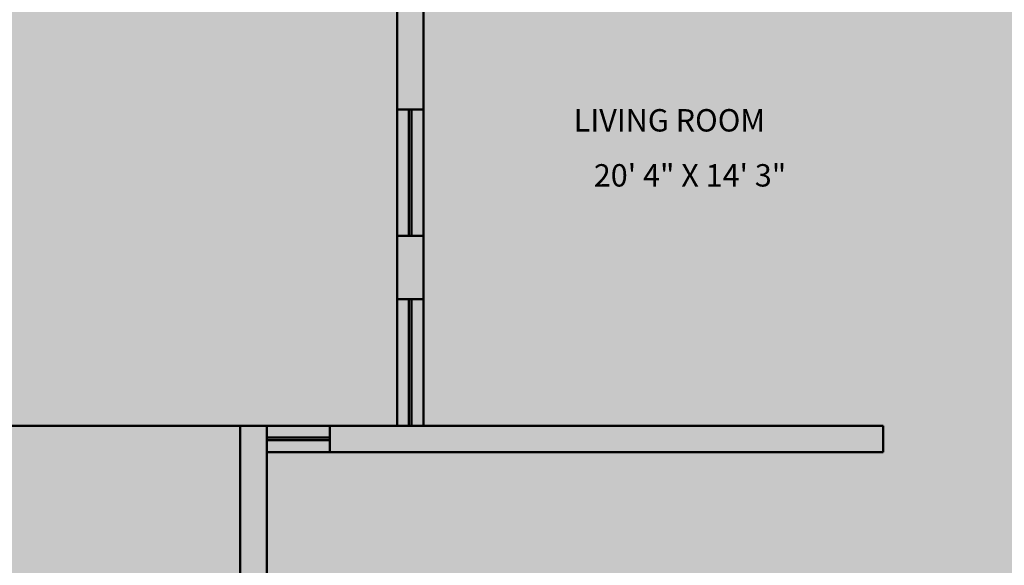
# Model space of a CAD drawing. Units: inches. Extents: x 925 to 2834, y 111 to 1355.
# Tile 4 of 25: x 1116 to 1490, y 675 to 882. Entities that reach past the tile are written whole.
import ezdxf

# ---------------------------------------------------------------- set-up
doc = ezdxf.new("R2010")
doc.units = ezdxf.units.IN
doc.header["$MEASUREMENT"] = 0
for name, color, linetype, lineweight in [('A-ANNO-DIMS', 2, 'Continuous', 18), ('A-AREA-IDEN', 7, 'Continuous', 18), ('A-FLOR-PATT', 252, 'Continuous', 13), ('A-WALL', 7, 'Continuous', 50), ('A-WALL-PATT', 8, 'Continuous', 13)]:
    doc.layers.add(name, color=color, linetype=linetype, lineweight=lineweight)
doc.styles.get("Standard").update_dxf_attribs({"font": 'arial.ttf'})
doc.dimstyles.get("Standard").update_dxf_attribs({"dimtxt": 6, "dimasz": 3, "dimexe": 0.18, "dimexo": 0.0625, "dimgap": 0.09, "dimtad": 0, "dimtih": 1, "dimtoh": 1, "dimdec": 1, "dimzin": 0, "dimdsep": 46, "dimlunit": 3, "dimtxsty": 'Standard', "dimblk": 'ARCHTICK', "dimcen": 0.09, "dimadec": 0, "dimazin": 0, "dimtfac": 1, "dimtdec": 1, "dimtofl": 0, "dimtmove": 0, "dimatfit": 3, "dimfxl": 1, "dimtolj": 1, "dimtzin": 0, "dimarcsym": 0})

# ---------------------------------------------------------------- blocks, each defined once
blk = doc.blocks.new('_ArchTick')
at = {"color": 0, "linetype": 'ByBlock', "const_width": 0.15}
blk.add_lwpolyline([(-0.5, -0.5), (0.5, 0.5)], dxfattribs=at)
blk = doc.blocks.new('*D25')
at = {"layer": 'A-ANNO-DIMS', "color": 0, "lineweight": -2, "transparency": 16777216}
for p, q in [((1200.21, 727.53), (1200.21, 115.18)), ((1084.71, 265.03), (1084.71, 115.18)), ((1084.71, 115.36), (1132.51, 115.36)), ((1200.21, 115.36), (1152.42, 115.36))]:
    blk.add_line(p, q, dxfattribs=at)
at = {"layer": 'Defpoints', "color": 0, "transparency": 16777216}
for p in [(1200.21, 727.59), (1084.71, 265.09), (1200.21, 115.36)]:
    blk.add_point(p, dxfattribs=at)
at = {"layer": 'A-ANNO-DIMS', "color": 0, "lineweight": -2, "transparency": 16777216, "xscale": 3, "yscale": 3, "zscale": 3, "rotation": 180}
blk.add_blockref('_ArchTick', (1084.71, 115.36), dxfattribs=at)
at = {"layer": 'A-ANNO-DIMS', "color": 0, "lineweight": -2, "transparency": 16777216, "xscale": 3, "yscale": 3, "zscale": 3}
blk.add_blockref('_ArchTick', (1200.21, 115.36), dxfattribs=at)
at = {"layer": 'A-ANNO-DIMS', "color": 0, "transparency": 16777216, "insert": (1142.46, 115.36), "char_height": 6, "attachment_point": 5}
blk.add_mtext('\\A1;115.5', dxfattribs=at)
blk = doc.blocks.new('*D26')
at = {"layer": 'A-ANNO-DIMS', "color": 0, "lineweight": -2, "transparency": 16777216}
for p, q in [((1200.21, 727.53), (1200.21, 115.18)), ((1434.21, 385.03), (1434.21, 115.18)), ((1200.21, 115.36), (1310.46, 115.36)), ((1434.21, 115.36), (1323.97, 115.36))]:
    blk.add_line(p, q, dxfattribs=at)
at = {"layer": 'Defpoints', "color": 0, "transparency": 16777216}
for p in [(1200.21, 727.59), (1434.21, 385.09), (1434.21, 115.36)]:
    blk.add_point(p, dxfattribs=at)
at = {"layer": 'A-ANNO-DIMS', "color": 0, "lineweight": -2, "transparency": 16777216, "xscale": 3, "yscale": 3, "zscale": 3, "rotation": 180}
blk.add_blockref('_ArchTick', (1200.21, 115.36), dxfattribs=at)
at = {"layer": 'A-ANNO-DIMS', "color": 0, "lineweight": -2, "transparency": 16777216, "xscale": 3, "yscale": 3, "zscale": 3}
blk.add_blockref('_ArchTick', (1434.21, 115.36), dxfattribs=at)
at = {"layer": 'A-ANNO-DIMS', "color": 0, "transparency": 16777216, "insert": (1317.21, 115.36), "char_height": 6, "attachment_point": 5}
blk.add_mtext('\\A1;234', dxfattribs=at)

msp = doc.modelspace()

# ---------------------------------------------------------------- hatches: boundary and pattern name
at = {"layer": 'A-FLOR-PATT', "transparency": 33554605}
h = msp.add_hatch(color=256, dxfattribs=at)
h.dxf.hatch_style = 1
h.paths.add_polyline_path([(1931.688, 1294.5638), (991.7375, 1294.5638), (991.7375, 172.1134), (1931.688, 172.1134)])
h.paths.add_polyline_path([(1910.7128, 1273.5886), (1910.7128, 193.0886), (1012.7128, 193.0886), (1012.7128, 1273.5886)], flags=16)
h.paths.add_polyline_path([(1850.7128, 1213.5886), (1850.7128, 253.0886), (1072.7128, 253.0886), (1072.7128, 1213.5886)], flags=0)
h.paths.add_polyline_path([(1838.7128, 1201.5886), (1838.7128, 265.0886), (1084.7128, 265.0886), (1084.7128, 530.5886), (1084.7128, 1201.5886)], flags=0)
h.paths.add_polyline_path([(1547.6758, 1155.7396), (1547.6758, 1119.115), (1513.0687, 1119.115), (1513.0687, 1155.7396)], flags=0)
h.paths.add_polyline_path([(1600.1067, 1154.9439), (1634.7139, 1154.9439), (1634.7139, 1119.115), (1600.1067, 1119.115)], flags=0)
h.paths.add_polyline_path([(1505.2502, 1144.5358), (1505.2502, 1119.115), (1470.643, 1119.115), (1470.643, 1144.5358)], flags=0)
h.paths.add_polyline_path([(1559.1357, 1141.0962), (1593.7428, 1141.0962), (1593.7428, 1119.115), (1559.1357, 1119.115)], flags=0)
h.paths.add_polyline_path([(1462.8966, 1154.9439), (1462.8966, 1119.115), (1428.2895, 1119.115), (1428.2895, 1154.9439)], flags=0)
h.paths.add_polyline_path([(1642.4603, 1144.5358), (1677.0675, 1144.5358), (1677.0675, 1119.115), (1642.4603, 1119.115)], flags=0)
h.paths.add_polyline_path([(1422.3508, 1141.0962), (1422.3508, 1119.115), (1387.7436, 1119.115), (1387.7436, 1141.0962)], flags=0)
h.paths.add_polyline_path([(1684.8859, 1155.7396), (1719.4931, 1155.7396), (1719.4931, 1119.115), (1684.8859, 1119.115)], flags=0)
h.paths.add_polyline_path([(1718.7128, 1081.5886), (1718.7128, 1050.1249), (1715.7128, 1050.1249), (1715.7128, 1026.1249), (1715.7128, 1002.1249), (1718.7128, 1002.1249), (1730.7128, 1002.1249), (1730.7128, 998.1249), (1730.7128, 990.1249), (1730.7128, 986.1249), (1718.7128, 986.1249), (1718.7128, 893.5886), (1715.3735, 893.5886), (1715.3735, 891.5886), (1713.3735, 891.5886, 0.41421356), (1677.3735, 855.5886), (1713.3735, 855.5886), (1713.3735, 853.5886), (1715.3735, 853.5886), (1715.3735, 851.5886), (1718.7128, 851.5886), (1718.7128, 821.5865), (1734.4655, 821.5865), (1734.3735, 819.5886, -0.41421356), (1712.4415, 793.5886), (1712.4415, 791.5886), (1718.7128, 791.5886), (1718.7128, 717.5886), (1718.7128, 669.5886), (1732.7128, 669.5886), (1732.7128, 665.5886), (1732.7128, 641.5886), (1732.7128, 634.5886), (1732.7128, 610.5886), (1732.7128, 603.5886), (1718.7128, 603.5886), (1718.7128, 385.0886), (1434.2128, 385.0886), (1434.2128, 530.5886), (1410.2128, 530.5886), (1408.2128, 530.5886), (1408.2128, 532.5886, 0.41421356), (1372.2128, 568.5886), (1372.2128, 532.5886), (1370.2128, 532.5886), (1370.2128, 530.5886), (1368.2128, 530.5886), (1282.2128, 530.5886), (1210.2128, 530.5886), (1200.2128, 530.5886), (1200.2128, 542.1915), (1183.2307, 542.1915), (1183.2307, 546.1915), (1200.2128, 546.1915), (1200.2128, 572.1915), (1183.2307, 572.1915), (1183.2307, 576.1915), (1200.2128, 576.1915), (1200.2128, 727.5886), (1210.2128, 727.5886), (1234.2128, 727.5886), (1259.7128, 727.5886), (1259.7128, 775.5886), (1259.7128, 799.5886), (1259.7128, 847.5886), (1259.7128, 993.5872), (1259.7128, 1065.5872), (1259.7128, 1071.5886), (1219.6318, 1071.5886), (1219.6318, 1081.5886), (1084.7128, 1081.5886), (1084.7128, 1119.115), (1256.8974, 1119.115), (1256.8974, 1154.9439), (1291.5046, 1154.9439), (1291.5046, 1119.115), (1256.8974, 1119.115), (1256.6723, 1081.5886), (1293.7128, 1081.5886), (1341.7128, 1081.5886), (1341.7128, 1093.5886), (1347.7128, 1093.5886), (1371.7128, 1093.5886), (1377.7128, 1093.5886), (1377.7128, 1081.5886), (1668.7128, 1081.5886), (1668.7128, 1117.5886), (1675.7128, 1117.5886), (1711.7128, 1117.5886), (1718.7128, 1117.5886)], flags=0)
h.paths.add_polyline_path([(1376.2838, 1155.7396), (1376.2838, 1119.115), (1341.6766, 1119.115), (1341.6766, 1155.7396)], flags=0)
h.paths.add_polyline_path([(1341.7128, 1076.0886), (1293.7128, 1076.0886), (1293.7128, 1071.5886), (1269.7128, 1071.5886), (1269.7128, 1065.5872), (1266.7128, 1065.5872), (1266.7128, 1029.5872), (1265.7128, 1029.5872), (1265.7128, 993.5872), (1269.7128, 993.5872), (1269.7128, 903.5886), (1269.7128, 893.5886), (1269.7128, 847.5886), (1265.2128, 847.5886), (1265.2128, 799.5886), (1269.7128, 799.5886), (1269.7128, 775.5886), (1265.2128, 775.5886), (1265.2128, 727.5886), (1269.7128, 727.5886), (1444.2128, 727.5886), (1444.2128, 717.5886), (1234.2128, 717.5886), (1234.2128, 722.0886), (1210.2128, 722.0886), (1210.2128, 717.5886), (1210.2128, 540.5886), (1210.2128, 536.0886), (1282.2128, 536.0886), (1282.2128, 535.0886), (1210.2128, 535.0886), (1210.2128, 540.5886), (1210.2128, 717.5886), (1210.2128, 723.0886), (1234.2128, 723.0886), (1234.2128, 717.5886), (1444.2128, 717.5886), (1444.2128, 727.5886), (1269.7128, 727.5886), (1264.2128, 727.5886), (1264.2128, 775.5886), (1269.7128, 775.5886), (1269.7128, 799.5886), (1264.2128, 799.5886), (1264.2128, 847.5886), (1269.7128, 847.5886), (1269.7128, 893.5886), (1269.7128, 903.5886), (1269.7128, 993.5872), (1264.7128, 993.5872), (1264.7128, 1029.5872), (1265.7128, 1029.5872), (1265.7128, 1065.5872), (1269.7128, 1065.5872), (1269.7128, 1071.5886), (1293.7128, 1071.5886), (1293.7128, 1077.0886), (1341.7128, 1077.0886)], flags=0)
h.paths.add_polyline_path([(1730.9529, 1141.0962), (1765.5601, 1141.0962), (1765.5601, 1119.115), (1730.9529, 1119.115)], flags=0)
h.paths.add_polyline_path([(1333.8582, 1144.5358), (1333.8582, 1119.115), (1299.251, 1119.115), (1299.251, 1144.5358)], flags=0)
h.paths.add_polyline_path([(1592.7128, 968.5886), (1596.0342, 968.5886), (1602.7128, 968.5886), (1708.7128, 968.5886), (1708.7128, 903.5886), (1602.7128, 903.5886), (1602.7128, 938.5886), (1592.7128, 938.5886), (1592.7128, 903.5886), (1451.7128, 903.5886), (1451.7128, 893.5886), (1511.7128, 893.5886), (1511.7128, 881.5886), (1515.2128, 881.5886), (1518.7128, 881.5886), (1518.7128, 893.5886), (1592.7128, 893.5886), (1592.7128, 799.5886), (1518.7128, 799.5886), (1518.7128, 857.5886), (1511.7128, 857.5886), (1511.7128, 799.5886), (1511.7128, 772.0886), (1521.7128, 772.0886), (1521.7128, 792.5886), (1592.7128, 792.5886), (1592.7128, 727.5886), (1521.7128, 727.5886), (1521.7128, 748.0886), (1511.7128, 748.0886), (1511.7128, 717.5886), (1708.7128, 717.5886), (1714.2128, 717.5886), (1714.2128, 669.5886), (1708.7128, 669.5886), (1708.7128, 641.5886), (1492.2128, 641.5886), (1492.2128, 631.5886), (1621.2128, 631.5886), (1621.2128, 443.0886), (1625.7128, 443.0886), (1625.7128, 503.0886), (1625.7128, 507.5886), (1625.7128, 631.5886), (1708.7128, 631.5886), (1708.7128, 507.5886), (1655.7128, 507.5886), (1655.7128, 503.0886), (1708.7128, 503.0886), (1708.7128, 395.0886), (1625.7128, 395.0886), (1625.7128, 419.0886), (1621.2128, 419.0886), (1621.2128, 395.0886), (1482.2128, 395.0886), (1482.2128, 385.0886), (1434.2128, 385.0886), (1434.2128, 433.0886), (1444.2128, 433.0886), (1444.2128, 631.5886), (1450.2128, 631.5886), (1450.2128, 634.91), (1452.2128, 634.91), (1452.2128, 669.5886), (1454.2128, 669.5886, -0.40021217), (1490.1712, 635.3173), (1492.2128, 635.3173), (1492.2128, 641.5886), (1564.7128, 641.5886), (1564.7128, 677.5886), (1672.7128, 677.5886), (1672.7128, 681.5886), (1564.7128, 681.5886), (1564.7128, 717.5886), (1511.7128, 717.5886), (1511.7128, 748.0886), (1511.7128, 772.0886), (1511.7128, 799.5886), (1511.7128, 857.5886), (1511.8913, 857.5886), (1511.8913, 859.5886), (1515.6201, 859.5886, 0.41421356), (1537.552, 879.5886), (1513.552, 879.5886), (1511.8913, 879.5886), (1511.8913, 881.5886), (1511.7128, 881.5886), (1511.7128, 893.5886), (1451.7128, 893.5886), (1451.7128, 903.5886), (1592.7128, 903.5886), (1592.7128, 938.5886), (1592.7128, 940.5886), (1596.4415, 940.5886, 0.41421356), (1618.3735, 966.5886), (1594.3735, 966.5886), (1592.7128, 966.5886)], flags=0)
h.paths.add_polyline_path([(1377.7128, 903.5886), (1377.7128, 893.5886), (1305.7128, 893.5886), (1305.7128, 903.5886)], flags=0)
h.paths.add_polyline_path([(1708.7128, 821.5886), (1712.0342, 821.5886), (1712.0342, 819.5886), (1710.3735, 819.5886), (1708.7128, 819.5886)], flags=0)
h.paths.add_polyline_path([(1576.7128, 695.1992), (1575.5896, 693.6649), (1575.9687, 694.6994), (1575.4438, 695.1992), (1575.9687, 695.699), (1575.5896, 696.7335)], flags=0)
h.paths.add_polyline_path([(1565.9817, 662.3134), (1565.4568, 661.8136), (1565.8359, 660.7791), (1564.7128, 662.3134), (1565.8359, 663.8477), (1565.4568, 662.8132)], flags=0)
h.paths.add_polyline_path([(1444.2128, 433.0886), (1444.2128, 395.0886), (1482.2128, 395.0886), (1482.2128, 389.0886), (1438.2128, 389.0886), (1438.2128, 391.8608), (1438.2128, 433.0886)], flags=0)
h.paths.add_polyline_path([(1410.2128, 506.5886), (1410.2128, 289.0886), (1108.7128, 289.0886), (1108.7128, 506.5886)], flags=0)
h.paths.add_polyline_path([(1612.3153, 838.3016), (1680.4151, 838.3016), (1680.4151, 851.3131), (1612.3153, 851.3131)], flags=8)
h.paths.add_polyline_path([(1208.3174, 395.0436), (1282.1017, 395.0436), (1282.1017, 408.0552), (1208.3174, 408.0552)], flags=8)
h.paths.add_polyline_path([(1291.8049, 598.7427), (1369.8017, 598.7427), (1369.8017, 611.7542), (1291.8049, 611.7542)], flags=8)
h.paths.add_polyline_path([(1119.679, 917.3022), (1191.0817, 917.3022), (1191.0817, 930.3137), (1119.679, 930.3137)], flags=8)
h.paths.add_polyline_path([(1332.2261, 815.9808), (1410.2258, 815.9808), (1410.2258, 829.001), (1332.2261, 829.001)], flags=8)
h.paths.add_polyline_path([(1390.9013, 955.8158), (1475.4981, 955.8158), (1475.4981, 968.8273), (1390.9013, 968.8273)], flags=8)
h.paths.add_polyline_path([(1620.3436, 998.9325), (1688.4434, 998.9325), (1688.4434, 1011.944), (1620.3436, 1011.944)], flags=8)
h.paths.add_polyline_path([(1620.3436, 914.1039), (1691.7405, 914.1039), (1691.7405, 927.1155), (1620.3436, 927.1155)], flags=8)
h.paths.add_polyline_path([(1521.4542, 816.005), (1589.5569, 816.005), (1589.5569, 829.0253), (1521.4542, 829.0253)], flags=8)
h.paths.add_polyline_path([(1528.524, 740.3497), (1602.3082, 740.3497), (1602.3082, 753.3613), (1528.524, 753.3613)], flags=8)
h.paths.add_polyline_path([(1627.6094, 762.6128), (1702.3091, 762.6128), (1702.3091, 775.6244), (1627.6094, 775.6244)], flags=8)
h.paths.add_polyline_path([(1610.5442, 657.2751), (1684.3284, 657.2751), (1684.3284, 670.2867), (1610.5442, 670.2867)], flags=8)
h.paths.add_polyline_path([(1636.6983, 519.472), (1711.3981, 519.472), (1711.3981, 532.4835), (1636.6983, 532.4835)], flags=8)
h.paths.add_polyline_path([(1616.8577, 424.8539), (1694.8545, 424.8539), (1694.8545, 437.8654), (1616.8577, 437.8654)], flags=8)
h.paths.add_polyline_path([(1506.1456, 460.8838), (1579.9299, 460.8838), (1579.9299, 473.8953), (1506.1456, 473.8953)], flags=8)
h.paths.add_polyline_path([(1624.6119, 784.6011), (1696.9185, 784.6011), (1696.9185, 797.7864), (1624.6119, 797.7864)], flags=8)
h.paths.add_polyline_path([(1606.3732, 854.2194), (1683.3039, 854.2194), (1683.3039, 867.4048), (1606.3732, 867.4048)], flags=8)
h.paths.add_polyline_path([(1127.8008, 940.3581), (1165.1637, 940.3581), (1165.1637, 953.5348), (1127.8008, 953.5348)], flags=8)
h.paths.add_polyline_path([(1620.8657, 1019.4968), (1677.3447, 1019.4968), (1677.3447, 1032.6735), (1620.8657, 1032.6735)], flags=8)
h.paths.add_polyline_path([(1620.8643, 930.1821), (1703.0564, 930.1821), (1703.0564, 943.3675), (1620.8643, 943.3675)], flags=8)
h.paths.add_polyline_path([(1324.5702, 836.8338), (1408.0892, 836.8338), (1408.0892, 850.0191), (1324.5702, 850.0191)], flags=8)
h.paths.add_polyline_path([(1281.6584, 622.8885), (1383.6213, 622.8885), (1383.6213, 636.0739), (1281.6584, 636.0739)], flags=8)
h.paths.add_polyline_path([(1210.6721, 416.7893), (1269.1299, 416.7893), (1269.1299, 429.9747), (1210.6721, 429.9747)], flags=8)
h.paths.add_polyline_path([(1507.8264, 477.4836), (1586.7329, 477.4836), (1586.7329, 490.669), (1507.8264, 490.669)], flags=8)
h.paths.add_polyline_path([(1643.6238, 443.8135), (1696.6696, 443.8135), (1696.6696, 456.5643), (1643.6238, 456.5643)], flags=8)
h.paths.add_polyline_path([(1647.2466, 540.5638), (1693.1825, 540.5638), (1693.1825, 553.7491), (1647.2466, 553.7491)], flags=8)
h.paths.add_polyline_path([(1626.0633, 668.5064), (1673.3174, 668.5064), (1673.3174, 681.6831), (1626.0633, 681.6831)], flags=8)
h.paths.add_polyline_path([(1538.2915, 830.7872), (1567.5942, 830.7872), (1567.5942, 843.5293), (1538.2915, 843.5293)], flags=8)
h.paths.add_polyline_path([(1530.9338, 754.0477), (1559.576, 754.0477), (1559.576, 766.7898), (1530.9338, 766.7898)], flags=8)
h.paths.add_polyline_path([(1351.2461, 979.2309), (1513.8919, 979.2309), (1513.8919, 992.4076), (1351.2461, 992.4076)], flags=8)
at = {"layer": 'A-FLOR-PATT'}
h = msp.add_hatch(color=256, dxfattribs=at)
h.dxf.hatch_style = 1
h.paths.add_polyline_path([(1850.7128, 1213.5886), (1072.7128, 1213.5886), (1072.7128, 253.0886), (1850.7128, 253.0886)])
h.paths.add_polyline_path([(1084.7128, 1201.5886), (1838.7128, 1201.5886), (1838.7128, 265.0886), (1084.7128, 265.0886)], flags=16)
h.paths.add_polyline_path([(1183.2307, 576.1915), (1200.2128, 576.1915), (1200.2128, 727.5886), (1210.2128, 727.5886), (1234.2128, 727.5886), (1259.7128, 727.5886), (1259.7128, 775.5886), (1259.7128, 799.5886), (1259.7128, 847.5886), (1259.7128, 993.5872), (1259.7128, 1065.5872), (1259.7128, 1071.5886), (1219.6318, 1071.5886), (1219.6318, 1081.5886), (1293.7128, 1081.5886), (1341.7128, 1081.5886), (1341.7128, 1093.5886), (1347.7128, 1093.5886), (1347.7128, 1081.5886), (1371.7128, 1081.5886), (1371.7128, 1093.5886), (1377.7128, 1093.5886), (1377.7128, 1081.5886), (1668.7128, 1081.5886), (1668.7128, 1117.5886), (1675.7128, 1117.5886), (1675.7128, 1081.5886), (1711.7128, 1081.5886), (1711.7128, 1117.5886), (1718.7128, 1117.5886), (1718.7128, 1081.5886), (1718.7128, 1050.1249), (1715.7128, 1050.1249), (1715.7128, 1026.1249), (1715.7128, 1002.1249), (1718.7128, 1002.1249), (1730.7128, 1002.1249), (1730.7128, 998.1249), (1730.7128, 990.1249), (1730.7128, 986.1249), (1718.7128, 986.1249), (1718.7128, 893.5886), (1715.3735, 893.5886), (1715.3735, 891.5886), (1713.3735, 891.5886, 0.41421356), (1677.3735, 855.5886), (1713.3735, 855.5886), (1713.3735, 853.5886), (1715.3735, 853.5886), (1715.3735, 851.5886), (1718.7128, 851.5886), (1718.7128, 821.5865), (1734.4655, 821.5865), (1734.3735, 819.5886, -0.41421356), (1712.4415, 793.5886), (1712.4415, 791.5886), (1718.7128, 791.5886), (1718.7128, 717.5886), (1718.7128, 669.5886), (1732.7128, 669.5886), (1732.7128, 665.5886), (1732.7128, 641.5886), (1732.7128, 634.5886), (1732.7128, 610.5886), (1732.7128, 603.5886), (1718.7128, 603.5886), (1718.7128, 385.0886), (1434.2128, 385.0886), (1434.2128, 433.0886), (1434.2128, 530.5886), (1410.2128, 530.5886), (1408.2128, 530.5886), (1408.2128, 532.5886, 0.41421356), (1372.2128, 568.5886), (1372.2128, 532.5886), (1370.2128, 532.5886), (1370.2128, 530.5886), (1368.2128, 530.5886), (1282.2128, 530.5886), (1210.2128, 530.5886), (1200.2128, 530.5886), (1200.2128, 542.1915), (1183.2307, 542.1915), (1183.2307, 546.1915), (1200.2128, 546.1915), (1200.2128, 572.1915), (1183.2307, 572.1915)], flags=0)
h.paths.add_polyline_path([(1210.2128, 717.5886), (1210.2128, 723.0886), (1234.2128, 723.0886), (1234.2128, 717.5886), (1444.2128, 717.5886), (1444.2128, 727.5886), (1269.7128, 727.5886), (1264.2128, 727.5886), (1264.2128, 775.5886), (1269.7128, 775.5886), (1269.7128, 799.5886), (1264.2128, 799.5886), (1264.2128, 847.5886), (1269.7128, 847.5886), (1269.7128, 893.5886), (1269.7128, 903.5886), (1269.7128, 993.5872), (1264.7128, 993.5872), (1264.7128, 1029.5872), (1265.7128, 1029.5872), (1265.7128, 1065.5872), (1269.7128, 1065.5872), (1269.7128, 1071.5886), (1293.7128, 1071.5886), (1293.7128, 1077.0886), (1341.7128, 1077.0886), (1341.7128, 1076.0886), (1293.7128, 1076.0886), (1293.7128, 1071.5886), (1269.7128, 1071.5886), (1269.7128, 1065.5872), (1266.7128, 1065.5872), (1266.7128, 1029.5872), (1265.7128, 1029.5872), (1265.7128, 993.5872), (1269.7128, 993.5872), (1269.7128, 903.5886), (1269.7128, 893.5886), (1269.7128, 847.5886), (1265.2128, 847.5886), (1265.2128, 799.5886), (1269.7128, 799.5886), (1269.7128, 775.5886), (1265.2128, 775.5886), (1265.2128, 727.5886), (1269.7128, 727.5886), (1444.2128, 727.5886), (1444.2128, 717.5886), (1234.2128, 717.5886), (1234.2128, 722.0886), (1210.2128, 722.0886), (1210.2128, 717.5886), (1210.2128, 540.5886), (1210.2128, 536.0886), (1282.2128, 536.0886), (1282.2128, 535.0886), (1210.2128, 535.0886), (1210.2128, 540.5886)], flags=0)
h.paths.add_polyline_path([(1450.2128, 634.91), (1452.2128, 634.91), (1452.2128, 669.5886), (1454.2128, 669.5886, -0.40021217), (1490.1712, 635.3173), (1492.2128, 635.3173), (1492.2128, 641.5886), (1564.7128, 641.5886), (1564.7128, 677.5886), (1672.7128, 677.5886), (1672.7128, 681.5886), (1564.7128, 681.5886), (1564.7128, 717.5886), (1511.7128, 717.5886), (1511.7128, 748.0886), (1511.7128, 772.0886), (1511.7128, 799.5886), (1511.7128, 857.5886), (1511.8913, 857.5886), (1511.8913, 859.5886), (1515.6201, 859.5886, 0.41421356), (1537.552, 879.5886), (1513.552, 879.5886), (1511.8913, 879.5886), (1511.8913, 881.5886), (1511.7128, 881.5886), (1511.7128, 893.5886), (1451.7128, 893.5886), (1451.7128, 903.5886), (1592.7128, 903.5886), (1592.7128, 938.5886), (1592.7128, 940.5886), (1596.4415, 940.5886, 0.41421356), (1618.3735, 966.5886), (1594.3735, 966.5886), (1592.7128, 966.5886), (1592.7128, 968.5886), (1596.0342, 968.5886), (1602.7128, 968.5886), (1708.7128, 968.5886), (1708.7128, 903.5886), (1602.7128, 903.5886), (1602.7128, 938.5886), (1592.7128, 938.5886), (1592.7128, 903.5886), (1451.7128, 903.5886), (1451.7128, 893.5886), (1511.7128, 893.5886), (1511.7128, 881.5886), (1518.7128, 881.5886), (1518.7128, 893.5886), (1592.7128, 893.5886), (1592.7128, 799.5886), (1518.7128, 799.5886), (1518.7128, 857.5886), (1511.7128, 857.5886), (1511.7128, 799.5886), (1511.7128, 772.0886), (1521.7128, 772.0886), (1521.7128, 792.5886), (1592.7128, 792.5886), (1592.7128, 727.5886), (1521.7128, 727.5886), (1521.7128, 748.0886), (1511.7128, 748.0886), (1511.7128, 717.5886), (1708.7128, 717.5886), (1714.2128, 717.5886), (1714.2128, 669.5886), (1708.7128, 669.5886), (1708.7128, 641.5886), (1492.2128, 641.5886), (1492.2128, 631.5886), (1621.2128, 631.5886), (1621.2128, 443.0886), (1625.7128, 443.0886), (1625.7128, 503.0886), (1625.7128, 507.5886), (1625.7128, 631.5886), (1708.7128, 631.5886), (1708.7128, 507.5886), (1655.7128, 507.5886), (1655.7128, 503.0886), (1708.7128, 503.0886), (1708.7128, 395.0886), (1625.7128, 395.0886), (1625.7128, 419.0886), (1621.2128, 419.0886), (1621.2128, 395.0886), (1482.2128, 395.0886), (1482.2128, 389.0886), (1438.2128, 389.0886), (1438.2128, 391.8608), (1438.2128, 433.0886), (1444.2128, 433.0886), (1444.2128, 631.5886), (1450.2128, 631.5886)], flags=0)
h.paths.add_polyline_path([(1444.2128, 433.0886), (1444.2128, 395.0886), (1482.2128, 395.0886), (1482.2128, 391.0886), (1440.2128, 391.0886), (1440.2128, 391.8608), (1440.2128, 433.0886)], flags=0)
h.paths.add_polyline_path([(1305.7128, 893.5886), (1305.7128, 903.5886), (1377.7128, 903.5886), (1377.7128, 893.5886)], flags=0)
h.paths.add_polyline_path([(1564.7128, 662.3134), (1565.8359, 663.8477), (1565.4568, 662.8132), (1565.9817, 662.3134), (1565.4568, 661.8136), (1565.8359, 660.7791)], flags=0)
h.paths.add_polyline_path([(1575.4438, 695.1992), (1575.9687, 695.699), (1575.5896, 696.7335), (1576.7128, 695.1992), (1575.5896, 693.6649), (1575.9687, 694.6994)], flags=0)
h.paths.add_polyline_path([(1708.7128, 821.5886), (1712.0342, 821.5886), (1712.0342, 819.5886), (1710.3735, 819.5886), (1708.7128, 819.5886)], flags=0)
h = msp.add_hatch(color=256, dxfattribs=at)
h.dxf.hatch_style = 1
h.paths.add_polyline_path([(1718.7128, 603.5886), (1708.7128, 603.5886), (1708.7128, 507.5886), (1655.7128, 507.5886), (1655.7128, 503.0886), (1708.7128, 503.0886), (1708.7128, 395.0886), (1625.7128, 395.0886), (1625.7128, 419.0886), (1621.2128, 419.0886), (1621.2128, 395.0886), (1482.2128, 395.0886), (1482.2128, 385.0886), (1718.7128, 385.0886)])
h.paths.add_polyline_path([(1625.7128, 631.5886), (1708.7128, 631.5886), (1708.7128, 603.5886), (1718.7128, 603.5886), (1732.7128, 603.5886), (1732.7128, 610.5886), (1715.7128, 610.5886), (1715.7128, 634.5886), (1732.7128, 634.5886), (1732.7128, 641.5886), (1715.7128, 641.5886), (1715.7128, 665.5886), (1732.7128, 665.5886), (1732.7128, 669.5886), (1708.7128, 669.5886), (1708.7128, 641.5886), (1492.2128, 641.5886), (1492.2128, 631.5886), (1621.2128, 631.5886), (1621.2128, 443.0886), (1625.7128, 443.0886), (1625.7128, 503.0886), (1625.7128, 507.5886)])
h.paths.add_polyline_path([(1718.7128, 851.5886), (1708.7128, 851.5886), (1708.7128, 828.5886), (1602.7128, 828.5886), (1602.7128, 893.5886), (1708.7128, 893.5886), (1718.7128, 893.5886), (1718.7128, 986.1249), (1730.7128, 986.1249), (1730.7128, 990.1249), (1718.7128, 990.1249), (1718.7128, 998.1249), (1730.7128, 998.1249), (1730.7128, 1002.1249), (1718.7128, 1002.1249), (1708.7128, 1002.1249), (1708.7128, 975.5886), (1602.7128, 975.5886), (1602.7128, 1011.5886), (1592.7128, 1011.5886), (1592.7128, 968.5886), (1596.0342, 968.5886), (1602.7128, 968.5886), (1708.7128, 968.5886), (1708.7128, 903.5886), (1602.7128, 903.5886), (1602.7128, 938.5886), (1592.7128, 938.5886), (1592.7128, 903.5886), (1451.7128, 903.5886), (1451.7128, 893.5886), (1511.7128, 893.5886), (1511.7128, 881.5886), (1515.2128, 881.5886), (1518.7128, 881.5886), (1518.7128, 893.5886), (1592.7128, 893.5886), (1592.7128, 799.5886), (1518.7128, 799.5886), (1518.7128, 857.5886), (1511.7128, 857.5886), (1511.7128, 799.5886), (1511.7128, 772.0886), (1521.7128, 772.0886), (1521.7128, 792.5886), (1592.7128, 792.5886), (1592.7128, 727.5886), (1521.7128, 727.5886), (1521.7128, 748.0886), (1511.7128, 748.0886), (1511.7128, 717.5886), (1708.7128, 717.5886), (1718.7128, 717.5886), (1718.7128, 727.5886), (1718.7128, 791.5886), (1708.7128, 791.5886), (1708.7128, 727.5886), (1602.7128, 727.5886), (1602.7128, 821.5886), (1708.7128, 821.5886), (1712.0342, 821.5886), (1718.7128, 821.5886)])
h.paths.add_polyline_path([(1718.7128, 1081.5886), (1718.7128, 1117.5886), (1711.7128, 1117.5886), (1711.7128, 1081.5886), (1675.7128, 1081.5886), (1675.7128, 1117.5886), (1668.7128, 1117.5886), (1668.7128, 1081.5886), (1377.7128, 1081.5886), (1377.7128, 1093.5886), (1371.7128, 1093.5886), (1371.7128, 1081.5886), (1347.7128, 1081.5886), (1347.7128, 1093.5886), (1341.7128, 1093.5886), (1341.7128, 1081.5886), (1341.7128, 1071.5886), (1592.7128, 1071.5886), (1592.7128, 1035.5886), (1602.7128, 1035.5886), (1602.7128, 1071.5886), (1708.7128, 1071.5886), (1708.7128, 1050.1249), (1718.7128, 1050.1249)])
h.paths.add_polyline_path([(1293.7128, 1081.5886), (1219.6318, 1081.5886), (1219.6318, 1071.5886), (1259.7128, 1071.5886), (1259.7128, 1065.5872), (1269.7128, 1065.5872), (1269.7128, 1071.5886), (1293.7128, 1071.5886)])
h.paths.add_polyline_path([(1269.7128, 903.5886), (1269.7128, 993.5872), (1259.7128, 993.5872), (1259.7128, 847.5886), (1269.7128, 847.5886), (1269.7128, 893.5886)])
h.paths.add_polyline_path([(1377.7128, 903.5886), (1305.7128, 903.5886), (1305.7128, 893.5886), (1377.7128, 893.5886)])
h.paths.add_polyline_path([(1444.2128, 727.5886), (1269.7128, 727.5886), (1259.7128, 727.5886), (1234.2128, 727.5886), (1234.2128, 717.5886), (1444.2128, 717.5886)])
h.paths.add_polyline_path([(1269.7128, 799.5886), (1259.7128, 799.5886), (1259.7128, 775.5886), (1269.7128, 775.5886)])
h.paths.add_polyline_path([(1444.2128, 631.5886), (1450.2128, 631.5886), (1450.2128, 634.91), (1450.2128, 641.5886), (1434.2128, 641.5886), (1434.2128, 540.5886), (1410.2128, 540.5886), (1410.2128, 530.5886), (1434.2128, 530.5886), (1434.2128, 433.0886), (1444.2128, 433.0886)])
h.paths.add_polyline_path([(1368.2128, 533.91), (1368.2128, 540.5886), (1282.2128, 540.5886), (1282.2128, 530.5886), (1368.2128, 530.5886)])
h.paths.add_polyline_path([(1210.2128, 717.5886), (1210.2128, 727.5886), (1200.2128, 727.5886), (1200.2128, 576.1915), (1183.2307, 576.1915), (1183.2307, 572.1915), (1200.2128, 572.1915), (1200.2128, 546.1915), (1183.2307, 546.1915), (1183.2307, 542.1915), (1200.2128, 542.1915), (1200.2128, 530.5886), (1210.2128, 530.5886), (1210.2128, 540.5886)])
at = {"layer": 'A-FLOR-PATT', "transparency": 33554574}
h = msp.add_hatch(color=256, dxfattribs=at)
h.dxf.hatch_style = 1
h.paths.add_polyline_path([(1259.7128, 993.5872), (1259.7128, 1065.5872), (1259.7128, 1071.5886), (1219.6318, 1071.5886), (1219.6318, 1081.5886), (1084.7128, 1081.5886), (1084.7128, 727.5886), (1200.2128, 727.5886), (1210.2128, 727.5886), (1234.2128, 727.5886), (1259.7128, 727.5886), (1259.7128, 775.5886), (1259.7128, 799.5886), (1259.7128, 847.5886)])
at = {"layer": 'A-FLOR-PATT', "transparency": 33554605}
h = msp.add_hatch(color=256, dxfattribs=at)
h.dxf.hatch_style = 1
h.paths.add_polyline_path([(1592.7128, 938.5886), (1592.7128, 940.5886), (1596.4415, 940.5886, 0.41421356), (1618.3735, 966.5886), (1594.3735, 966.5886), (1592.7128, 966.5886), (1592.7128, 968.5886), (1592.7128, 1011.5886), (1602.7128, 1011.5886), (1602.7128, 975.5886), (1708.7128, 975.5886), (1708.7128, 1002.1249), (1711.7128, 1002.1249), (1711.7128, 1026.1249), (1711.7128, 1050.1249), (1708.7128, 1050.1249), (1708.7128, 1071.5886), (1602.7128, 1071.5886), (1602.7128, 1035.5886), (1592.7128, 1035.5886), (1592.7128, 1071.5886), (1341.7128, 1071.5886), (1293.7128, 1071.5886), (1269.7128, 1071.5886), (1269.7128, 1065.5872), (1269.7128, 993.5872), (1269.7128, 903.5886), (1269.7128, 893.5886), (1269.7128, 847.5886), (1269.7128, 799.5886), (1269.7128, 775.5886), (1269.7128, 727.5886), (1444.2128, 727.5886), (1444.2128, 717.5886), (1234.2128, 717.5886), (1210.2128, 717.5886), (1210.2128, 540.5886), (1282.2128, 540.5886), (1368.2128, 540.5886), (1368.2128, 533.91), (1370.2128, 533.91), (1370.2128, 568.5886), (1372.2128, 568.5886, -0.40021217), (1408.1712, 534.3173), (1410.2128, 534.3173), (1410.2128, 540.5886), (1434.2128, 540.5886), (1434.2128, 641.5886), (1450.2128, 641.5886), (1450.2128, 634.91), (1452.2128, 634.91), (1452.2128, 669.5886), (1454.2128, 669.5886, -0.40021217), (1490.1712, 635.3173), (1492.2128, 635.3173), (1492.2128, 641.5886), (1564.7128, 641.5886), (1564.7128, 677.5886), (1672.7128, 677.5886), (1672.7128, 681.5886), (1564.7128, 681.5886), (1564.7128, 717.5886), (1511.7128, 717.5886), (1511.7128, 748.0886), (1511.7128, 772.0886), (1511.7128, 799.5886), (1511.7128, 857.5886), (1511.8913, 857.5886), (1511.8913, 859.5886), (1515.6201, 859.5886, 0.41421356), (1537.552, 879.5886), (1513.552, 879.5886), (1511.8913, 879.5886), (1511.8913, 881.5886), (1511.7128, 881.5886), (1511.7128, 893.5886), (1451.7128, 893.5886), (1451.7128, 903.5886), (1592.7128, 903.5886)])
h.paths.add_polyline_path([(1377.7128, 903.5886), (1377.7128, 893.5886), (1305.7128, 893.5886), (1305.7128, 903.5886)], flags=16)
h.paths.add_polyline_path([(1592.7128, 893.5886), (1518.7128, 893.5886), (1518.7128, 881.5865), (1537.6441, 881.5865), (1537.552, 879.5886, -0.41421356), (1515.6201, 859.5886), (1515.6201, 857.5886), (1518.7128, 857.5886), (1518.7128, 799.5886), (1592.7128, 799.5886)], flags=17)
h.paths.add_polyline_path([(1291.8049, 598.7427), (1369.8017, 598.7427), (1369.8017, 611.7542), (1291.8049, 611.7542)], flags=24)
h.paths.add_polyline_path([(1332.2261, 815.9808), (1410.2258, 815.9808), (1410.2258, 829.001), (1332.2261, 829.001)], flags=24)
h.paths.add_polyline_path([(1390.9013, 955.8158), (1475.4981, 955.8158), (1475.4981, 968.8273), (1390.9013, 968.8273)], flags=24)
h.paths.add_polyline_path([(1620.3436, 998.9325), (1688.4434, 998.9325), (1688.4434, 1011.944), (1620.3436, 1011.944)], flags=24)
h.paths.add_polyline_path([(1620.8657, 1019.4968), (1677.3447, 1019.4968), (1677.3447, 1032.6735), (1620.8657, 1032.6735)], flags=24)
h.paths.add_polyline_path([(1324.5702, 836.8338), (1408.0892, 836.8338), (1408.0892, 850.0191), (1324.5702, 850.0191)], flags=24)
h.paths.add_polyline_path([(1281.6584, 622.8885), (1383.6213, 622.8885), (1383.6213, 636.0739), (1281.6584, 636.0739)], flags=24)
h.paths.add_polyline_path([(1626.0633, 668.5064), (1673.3174, 668.5064), (1673.3174, 681.6831), (1626.0633, 681.6831)], flags=25)
h.paths.add_polyline_path([(1351.2461, 979.2309), (1513.8919, 979.2309), (1513.8919, 992.4076), (1351.2461, 992.4076)], flags=24)
h.paths.add_polyline_path([(1521.4542, 816.005), (1589.5569, 816.005), (1589.5569, 829.0253), (1521.4542, 829.0253)], flags=24)
h.paths.add_polyline_path([(1538.2915, 830.7872), (1567.5942, 830.7872), (1567.5942, 843.5293), (1538.2915, 843.5293)], flags=24)
h.paths.add_polyline_path([(1636.6983, 519.472), (1711.3981, 519.472), (1711.3981, 532.4835), (1636.6983, 532.4835)], flags=9)
h.paths.add_polyline_path([(1616.8577, 424.8539), (1694.8545, 424.8539), (1694.8545, 437.8654), (1616.8577, 437.8654)], flags=9)
h.paths.add_polyline_path([(1506.1456, 460.8838), (1579.9299, 460.8838), (1579.9299, 473.8953), (1506.1456, 473.8953)], flags=9)
h.paths.add_polyline_path([(1606.3732, 854.2194), (1683.3039, 854.2194), (1683.3039, 867.4048), (1606.3732, 867.4048)], flags=25)
h.paths.add_polyline_path([(1507.8264, 477.4836), (1586.7329, 477.4836), (1586.7329, 490.669), (1507.8264, 490.669)], flags=9)
h.paths.add_polyline_path([(1643.6238, 443.8135), (1696.6696, 443.8135), (1696.6696, 456.5643), (1643.6238, 456.5643)], flags=9)
h.paths.add_polyline_path([(1647.2466, 540.5638), (1693.1825, 540.5638), (1693.1825, 553.7491), (1647.2466, 553.7491)], flags=25)
h = msp.add_hatch(color=256, dxfattribs=at)
h.dxf.hatch_style = 1
h.paths.add_polyline_path([(1200.2128, 727.5886), (1084.7128, 727.5886), (1084.7128, 530.5886), (1200.2128, 530.5886), (1200.2128, 542.1915), (1183.2307, 542.1915), (1183.2307, 546.1915), (1200.2128, 546.1915), (1200.2128, 572.1915), (1183.2307, 572.1915), (1183.2307, 576.1915), (1200.2128, 576.1915)])
h.paths.add_polyline_path([(1612.3153, 838.3016), (1680.4151, 838.3016), (1680.4151, 851.3131), (1612.3153, 851.3131)], flags=9)
h.paths.add_polyline_path([(1291.8049, 598.7427), (1369.8017, 598.7427), (1369.8017, 611.7542), (1291.8049, 611.7542)], flags=9)
h.paths.add_polyline_path([(1119.679, 917.3022), (1191.0817, 917.3022), (1191.0817, 930.3137), (1119.679, 930.3137)], flags=9)
h.paths.add_polyline_path([(1332.2261, 815.9808), (1410.2258, 815.9808), (1410.2258, 829.001), (1332.2261, 829.001)], flags=9)
h.paths.add_polyline_path([(1390.9013, 955.8158), (1475.4981, 955.8158), (1475.4981, 968.8273), (1390.9013, 968.8273)], flags=9)
h.paths.add_polyline_path([(1620.3436, 998.9325), (1688.4434, 998.9325), (1688.4434, 1011.944), (1620.3436, 1011.944)], flags=9)
h.paths.add_polyline_path([(1620.3436, 914.1039), (1691.7405, 914.1039), (1691.7405, 927.1155), (1620.3436, 927.1155)], flags=9)
h.paths.add_polyline_path([(1521.4542, 816.005), (1589.5569, 816.005), (1589.5569, 829.0253), (1521.4542, 829.0253)], flags=9)
h.paths.add_polyline_path([(1522.4337, 740.3497), (1596.218, 740.3497), (1596.218, 753.3613), (1522.4337, 753.3613)], flags=9)
h.paths.add_polyline_path([(1606.3732, 854.2194), (1683.3039, 854.2194), (1683.3039, 867.4048), (1606.3732, 867.4048)], flags=9)
h.paths.add_polyline_path([(1127.8008, 940.3581), (1165.1637, 940.3581), (1165.1637, 953.5348), (1127.8008, 953.5348)], flags=9)
h.paths.add_polyline_path([(1620.8657, 1019.4968), (1677.3447, 1019.4968), (1677.3447, 1032.6735), (1620.8657, 1032.6735)], flags=9)
h.paths.add_polyline_path([(1620.8643, 930.1821), (1703.0564, 930.1821), (1703.0564, 943.3675), (1620.8643, 943.3675)], flags=9)
h.paths.add_polyline_path([(1324.5702, 836.8338), (1408.0892, 836.8338), (1408.0892, 850.0191), (1324.5702, 850.0191)], flags=9)
h.paths.add_polyline_path([(1281.6584, 622.8885), (1383.6213, 622.8885), (1383.6213, 636.0739), (1281.6584, 636.0739)], flags=9)
h.paths.add_polyline_path([(1626.0633, 668.5064), (1673.3174, 668.5064), (1673.3174, 681.6831), (1626.0633, 681.6831)], flags=9)
h.paths.add_polyline_path([(1538.2915, 830.7872), (1567.5942, 830.7872), (1567.5942, 843.5293), (1538.2915, 843.5293)], flags=9)
h.paths.add_polyline_path([(1351.2461, 979.2309), (1513.8919, 979.2309), (1513.8919, 992.4076), (1351.2461, 992.4076)], flags=9)
h = msp.add_hatch(color=256, dxfattribs=at)
h.dxf.hatch_style = 1
h.paths.add_polyline_path([(1621.2128, 631.5886), (1492.2128, 631.5886), (1490.2128, 631.5886), (1490.2128, 633.5886, 0.41421356), (1454.2128, 669.5886), (1454.2128, 633.5886), (1452.2128, 633.5886), (1452.2128, 631.5886), (1450.2128, 631.5886), (1444.2128, 631.5886), (1444.2128, 395.0886), (1482.2128, 395.0886), (1621.2128, 395.0886), (1621.2128, 419.0886), (1625.7128, 419.0886), (1625.7128, 395.0886), (1708.7128, 395.0886), (1708.7128, 503.0886), (1655.7128, 503.0886), (1655.7128, 507.5886), (1708.7128, 507.5886), (1708.7128, 631.5886), (1625.7128, 631.5886), (1625.7128, 507.5886), (1625.7128, 503.0886), (1625.7128, 443.0886), (1621.2128, 443.0886)])
h.paths.add_polyline_path([(1636.6983, 519.472), (1711.3981, 519.472), (1711.3981, 532.4835), (1636.6983, 532.4835)], flags=9)
h.paths.add_polyline_path([(1616.8577, 424.8539), (1694.8545, 424.8539), (1694.8545, 437.8654), (1616.8577, 437.8654)], flags=24)
h.paths.add_polyline_path([(1506.1456, 460.8838), (1579.9299, 460.8838), (1579.9299, 473.8953), (1506.1456, 473.8953)], flags=24)
h.paths.add_polyline_path([(1507.8264, 477.4836), (1586.7329, 477.4836), (1586.7329, 490.669), (1507.8264, 490.669)], flags=24)
h.paths.add_polyline_path([(1643.6238, 443.8135), (1696.6696, 443.8135), (1696.6696, 456.5643), (1643.6238, 456.5643)], flags=24)
h.paths.add_polyline_path([(1647.2466, 540.5638), (1693.1825, 540.5638), (1693.1825, 553.7491), (1647.2466, 553.7491)], flags=24)
h.paths.add_polyline_path([(1612.3153, 838.3016), (1680.4151, 838.3016), (1680.4151, 851.3131), (1612.3153, 851.3131)], flags=9)
h.paths.add_polyline_path([(1291.8049, 598.7427), (1369.8017, 598.7427), (1369.8017, 611.7542), (1291.8049, 611.7542)], flags=9)
h.paths.add_polyline_path([(1119.679, 917.3022), (1191.0817, 917.3022), (1191.0817, 930.3137), (1119.679, 930.3137)], flags=9)
h.paths.add_polyline_path([(1332.2261, 815.9808), (1410.2258, 815.9808), (1410.2258, 829.001), (1332.2261, 829.001)], flags=9)
h.paths.add_polyline_path([(1390.9013, 955.8158), (1475.4981, 955.8158), (1475.4981, 968.8273), (1390.9013, 968.8273)], flags=9)
h.paths.add_polyline_path([(1620.3436, 998.9325), (1688.4434, 998.9325), (1688.4434, 1011.944), (1620.3436, 1011.944)], flags=9)
h.paths.add_polyline_path([(1620.3436, 914.1039), (1691.7405, 914.1039), (1691.7405, 927.1155), (1620.3436, 927.1155)], flags=9)
h.paths.add_polyline_path([(1521.4542, 816.005), (1589.5569, 816.005), (1589.5569, 829.0253), (1521.4542, 829.0253)], flags=9)
h.paths.add_polyline_path([(1528.524, 740.3497), (1602.3082, 740.3497), (1602.3082, 753.3613), (1528.524, 753.3613)], flags=9)
h.paths.add_polyline_path([(1627.6094, 762.6128), (1702.3091, 762.6128), (1702.3091, 775.6244), (1627.6094, 775.6244)], flags=9)
h.paths.add_polyline_path([(1624.6119, 784.6011), (1696.9185, 784.6011), (1696.9185, 797.7864), (1624.6119, 797.7864)], flags=9)
h.paths.add_polyline_path([(1606.3732, 854.2194), (1683.3039, 854.2194), (1683.3039, 867.4048), (1606.3732, 867.4048)], flags=9)
h.paths.add_polyline_path([(1127.8008, 940.3581), (1165.1637, 940.3581), (1165.1637, 953.5348), (1127.8008, 953.5348)], flags=9)
h.paths.add_polyline_path([(1620.8657, 1019.4968), (1677.3447, 1019.4968), (1677.3447, 1032.6735), (1620.8657, 1032.6735)], flags=9)
h.paths.add_polyline_path([(1620.8643, 930.1821), (1703.0564, 930.1821), (1703.0564, 943.3675), (1620.8643, 943.3675)], flags=9)
h.paths.add_polyline_path([(1324.5702, 836.8338), (1408.0892, 836.8338), (1408.0892, 850.0191), (1324.5702, 850.0191)], flags=9)
h.paths.add_polyline_path([(1281.6584, 622.8885), (1383.6213, 622.8885), (1383.6213, 636.0739), (1281.6584, 636.0739)], flags=9)
h.paths.add_polyline_path([(1626.0633, 668.5064), (1673.3174, 668.5064), (1673.3174, 681.6831), (1626.0633, 681.6831)], flags=9)
h.paths.add_polyline_path([(1538.2915, 830.7872), (1567.5942, 830.7872), (1567.5942, 843.5293), (1538.2915, 843.5293)], flags=9)
h.paths.add_polyline_path([(1530.9338, 754.0477), (1559.576, 754.0477), (1559.576, 766.7898), (1530.9338, 766.7898)], flags=9)
h.paths.add_polyline_path([(1351.2461, 979.2309), (1513.8919, 979.2309), (1513.8919, 992.4076), (1351.2461, 992.4076)], flags=9)
at = {"layer": 'A-WALL-PATT'}
h = msp.add_hatch(color=256, dxfattribs=at)
h.dxf.hatch_style = 1
h.set_gradient(color1=(255, 255, 255), tint=1)
h.paths.add_polyline_path([(1269.7128, 799.5886), (1269.7128, 847.5886), (1265.2128, 847.5886), (1265.2128, 799.5886)])
h.paths.add_polyline_path([(1264.2128, 799.5886), (1264.2128, 847.5886), (1259.7128, 847.5886), (1259.7128, 799.5886)])
h = msp.add_hatch(color=256, dxfattribs=at)
h.dxf.hatch_style = 1
h.set_gradient(color1=(99, 100, 102), color2=(99, 100, 102), tint=1)
h.paths.add_polyline_path([(1265.2128, 799.5886), (1265.2128, 847.5886), (1264.2128, 847.5886), (1264.2128, 799.5886)])
h = msp.add_hatch(color=256, dxfattribs=at)
h.dxf.hatch_style = 1
h.set_gradient(color1=(255, 255, 255), tint=1)
h.paths.add_polyline_path([(1269.7128, 727.5886), (1269.7128, 775.5886), (1265.2128, 775.5886), (1265.2128, 727.5886)])
h.paths.add_polyline_path([(1264.2128, 727.5886), (1264.2128, 775.5886), (1259.7128, 775.5886), (1259.7128, 727.5886)])
h = msp.add_hatch(color=256, dxfattribs=at)
h.dxf.hatch_style = 1
h.set_gradient(color1=(99, 100, 102), color2=(99, 100, 102), tint=1)
h.paths.add_polyline_path([(1265.2128, 727.5886), (1265.2128, 775.5886), (1264.2128, 775.5886), (1264.2128, 727.5886)])
h = msp.add_hatch(color=256, dxfattribs=at)
h.dxf.hatch_style = 1
h.paths.add_polyline_path([(1234.2128, 723.0886), (1210.2128, 723.0886), (1210.2128, 722.0886), (1234.2128, 722.0886)], flags=17)
h.paths.add_polyline_path([(1234.2128, 727.5886), (1210.2128, 727.5886), (1210.2128, 723.0886), (1234.2128, 723.0886)])
h.paths.add_polyline_path([(1234.2128, 723.0886), (1210.2128, 723.0886), (1210.2128, 717.5886), (1234.2128, 717.5886)])
h = msp.add_hatch(color=256, dxfattribs=at)
h.dxf.hatch_style = 1
h.paths.add_polyline_path([(1234.2128, 723.0886), (1210.2128, 723.0886), (1210.2128, 722.0886), (1234.2128, 722.0886)])

# ---------------------------------------------------------------- linework, layer by layer
at = {"layer": 'A-WALL'}
for p, q in [((1259.7128, 993.5872), (1259.7128, 847.5886)), ((1269.7128, 893.5886), (1269.7128, 847.5886)), ((1269.7128, 847.5886), (1259.7128, 847.5886)), ((1264.2128, 847.5886), (1264.2128, 799.5886)), ((1265.2128, 847.5886), (1265.2128, 799.5886)), ((1269.7128, 799.5886), (1259.7128, 799.5886)), ((1259.7128, 799.5886), (1259.7128, 775.5886)), ((1269.7128, 799.5886), (1269.7128, 775.5886)), ((1269.7128, 775.5886), (1259.7128, 775.5886)), ((1264.2128, 775.5886), (1264.2128, 727.5886)), ((1265.2128, 775.5886), (1265.2128, 727.5886)), ((1200.2128, 727.5886), (1084.7128, 727.5886)), ((1200.2128, 727.5886), (1200.2128, 576.1915)), ((1200.2128, 727.5886), (1210.2128, 727.5886)), ((1210.2128, 717.5886), (1210.2128, 727.5886)), ((1259.7128, 727.5886), (1234.2128, 727.5886)), ((1234.2128, 717.5886), (1234.2128, 727.5886)), ((1269.7128, 727.5886), (1259.7128, 727.5886)), ((1444.2128, 727.5886), (1269.7128, 727.5886)), ((1444.2128, 727.5886), (1444.2128, 717.5886)), ((1210.2128, 723.0886), (1234.2128, 723.0886)), ((1210.2128, 722.0886), (1234.2128, 722.0886)), ((1210.2128, 717.5886), (1210.2128, 540.5886)), ((1444.2128, 717.5886), (1234.2128, 717.5886))]:
    msp.add_line(p, q, dxfattribs=at)
for points in [[(1269.7128, 847.5886), (1269.7128, 799.5886), (1259.7128, 799.5886), (1259.7128, 847.5886)], [(1269.7128, 775.5886), (1269.7128, 727.5886), (1259.7128, 727.5886), (1259.7128, 775.5886)], [(1234.2128, 717.5886), (1210.2128, 717.5886), (1210.2128, 727.5886), (1234.2128, 727.5886)]]:
    msp.add_lwpolyline(points, close=True, dxfattribs=at)

# ---------------------------------------------------------------- texts
at = {"layer": 'A-AREA-IDEN'}
for s, p in [('LIVING ROOM', (1326.7677, 839.1762)), ('20\' 4" X 14\' 3"', (1334.3961, 818.3015))]:
    msp.add_text(s, height=8.494735, dxfattribs=at).set_placement(p)

# ---------------------------------------------------------------- dimensions: what is measured, and where the dimension line sits
at = {"layer": 'A-ANNO-DIMS'}
for base, p1, p2, override, picture, middle in [((1200.2128, 115.3634), (1084.7128, 265.0886), (1200.2128, 727.5886), {"dimdec": 1, "dimlfac": 1, "dimrnd": 0, "dimzin": 0, "dimdsep": 46, "dimlunit": 2}, '*D25', (1142.4628, 115.3634)), ((1434.2128, 115.3634), (1200.2128, 727.5886), (1434.2128, 385.0886), {"dimdec": 0, "dimlfac": 1, "dimrnd": 0, "dimzin": 0, "dimdsep": 46, "dimlunit": 2}, '*D26', (1317.2128, 115.3634))]:
    dim = msp.add_linear_dim(base=base, p1=p1, p2=p2, dimstyle='Standard', override=override, dxfattribs=at)
    dim.commit()
    dim.dimension.update_dxf_attribs({"geometry": picture, "text_midpoint": middle})

doc.saveas('drawing.dxf')
